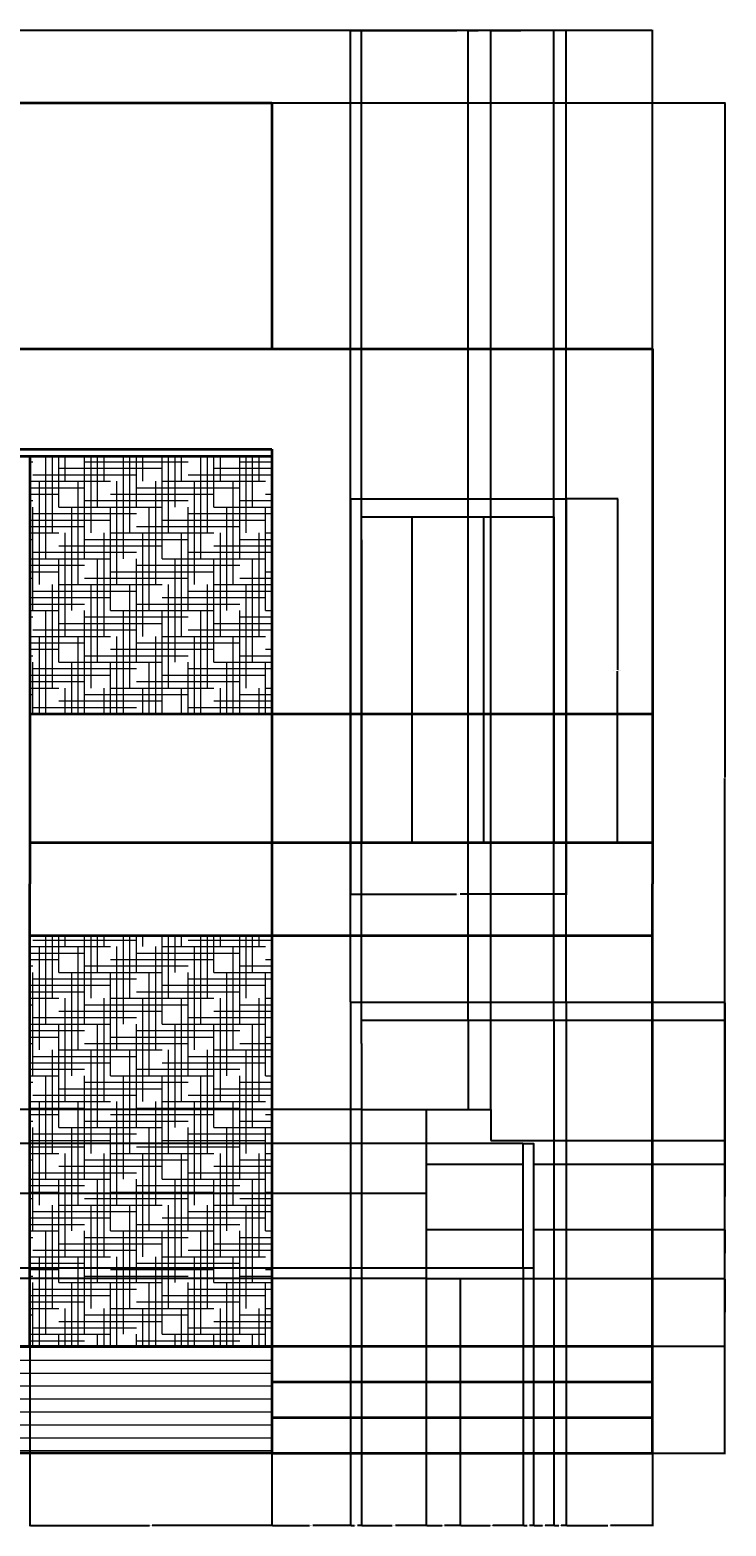
# Model space of a CAD drawing. Units: inches. Extents: x 18 to 448, y 19 to 438.
# Tile 2 of 2: x 253 to 448, y 19 to 438. Entities that reach past the tile are written whole.
import ezdxf

# ---------------------------------------------------------------- set-up
doc = ezdxf.new("R2010")
doc.units = ezdxf.units.IN
doc.header["$MEASUREMENT"] = 0
for name, color, linetype, lineweight in [('A-ANNO-DIMS', 2, 'Continuous', 18), ('A-DOOR', 3, 'Continuous', 25), ('A-ELEV', 7, 'Continuous', 35), ('A-ELEV-PATT', 8, 'Continuous', 13)]:
    doc.layers.add(name, color=color, linetype=linetype, lineweight=lineweight)
doc.styles.get("Standard").update_dxf_attribs({"font": 'arial.ttf'})
doc.dimstyles.get("Standard").update_dxf_attribs({"dimtxt": 0.18, "dimasz": 0.18, "dimexe": 0.18, "dimexo": 0.0625, "dimgap": 0.09, "dimtad": 0, "dimtih": 1, "dimtoh": 1, "dimdec": 4, "dimzin": 0, "dimdsep": 46, "dimtxsty": 'Standard', "dimcen": 0.09, "dimadec": 0, "dimazin": 0, "dimtfac": 1, "dimtdec": 4, "dimtofl": 0, "dimtmove": 0, "dimatfit": 3, "dimfxl": 1, "dimtolj": 1, "dimtzin": 0, "dimarcsym": 0})

# ---------------------------------------------------------------- blocks, each defined once
blk = doc.blocks.new('DOOR-FRAME')
for p, q in [((0, 96.46), (0, 4.77)), ((0, 96.46), (6.57, 96.46)), ((6.57, 96.46), (60.43, 96.46)), ((60.43, 96.46), (60.43, 0)), ((3.01, 84.89), (3.01, 91.39)), ((3.01, 91.39), (57.03, 91.39)), ((57.03, 91.39), (57.03, 84.89)), ((3.01, 84.89), (3.01, 0)), ((57.03, 84.89), (57.03, 0)), ((0, 4.77), (0, 0))]:
    blk.add_line(p, q)
blk = doc.blocks.new('*D5')
at = {"layer": 'A-ANNO-DIMS', "color": 0, "lineweight": -2, "transparency": 16777216}
for p, q in [((403.35, 306.87), (417.94, 306.87)), ((417.76, 306.69), (417.76, 258.82)), ((417.76, 210.58), (417.76, 258.45)), ((403.35, 210.4), (417.94, 210.4))]:
    blk.add_line(p, q, dxfattribs=at)
at = {"layer": 'A-ANNO-DIMS', "color": 0, "transparency": 16777216}
for points in [[(417.73, 306.69), (417.79, 306.69), (417.76, 306.87)], [(417.73, 210.58), (417.79, 210.58), (417.76, 210.4)]]:
    blk.add_solid(points, dxfattribs=at)
at = {"layer": 'Defpoints', "color": 0, "transparency": 16777216}
for p in [(403.29, 306.87), (417.76, 306.87), (403.29, 210.4)]:
    blk.add_point(p, dxfattribs=at)
at = {"layer": 'A-ANNO-DIMS', "color": 0, "transparency": 16777216, "insert": (417.76, 258.64), "char_height": 0.18, "attachment_point": 5}
blk.add_mtext('\\A1;DOOR FRAME 96 TYP.', dxfattribs=at)
blk = doc.blocks.new('*D6')
at = {"layer": 'A-ANNO-DIMS', "color": 0, "lineweight": -2, "transparency": 16777216}
for p, q in [((342.86, 210.34), (342.86, 195.76)), ((403.29, 210.34), (403.29, 195.76)), ((343.04, 195.94), (372.54, 195.94)), ((403.11, 195.94), (373.6, 195.94))]:
    blk.add_line(p, q, dxfattribs=at)
at = {"layer": 'A-ANNO-DIMS', "color": 0, "transparency": 16777216}
for points in [[(343.04, 195.97), (343.04, 195.91), (342.86, 195.94)], [(403.11, 195.97), (403.11, 195.91), (403.29, 195.94)]]:
    blk.add_solid(points, dxfattribs=at)
at = {"layer": 'Defpoints', "color": 0, "transparency": 16777216}
for p in [(342.86, 210.4), (403.29, 210.4), (403.29, 195.94)]:
    blk.add_point(p, dxfattribs=at)
at = {"layer": 'A-ANNO-DIMS', "color": 0, "transparency": 16777216, "insert": (373.07, 195.94), "char_height": 0.18, "attachment_point": 5}
blk.add_mtext('\\A1;60 TYP.', dxfattribs=at)
blk = doc.blocks.new('*D7')
at = {"layer": 'A-ANNO-DIMS', "color": 0, "lineweight": -2, "transparency": 16777216}
for p, q in [((38.85, 39.26), (38.85, 438.34)), ((39.03, 438.16), (232.72, 438.16)), ((427.33, 438.16), (233.64, 438.16)), ((427.51, 39.26), (427.51, 438.34))]:
    blk.add_line(p, q, dxfattribs=at)
at = {"layer": 'A-ANNO-DIMS', "color": 0, "transparency": 16777216}
for points in [[(39.03, 438.19), (39.03, 438.13), (38.85, 438.16)], [(427.33, 438.19), (427.33, 438.13), (427.51, 438.16)]]:
    blk.add_solid(points, dxfattribs=at)
at = {"layer": 'Defpoints', "color": 0, "transparency": 16777216}
for p in [(427.51, 438.16), (38.85, 39.19), (427.51, 39.19)]:
    blk.add_point(p, dxfattribs=at)
at = {"layer": 'A-ANNO-DIMS', "color": 0, "transparency": 16777216, "insert": (233.18, 438.16), "char_height": 0.18, "attachment_point": 5}
blk.add_mtext('\\A1;388.66', dxfattribs=at)
blk = doc.blocks.new('*D8')
at = {"layer": 'A-ANNO-DIMS', "color": 0, "lineweight": -2, "transparency": 16777216}
for p, q in [((320.8, 417.86), (447.99, 417.86)), ((447.81, 417.68), (447.81, 228.71)), ((447.81, 39.37), (447.81, 228.34)), ((427.57, 39.19), (447.99, 39.19))]:
    blk.add_line(p, q, dxfattribs=at)
at = {"layer": 'A-ANNO-DIMS', "color": 0, "transparency": 16777216}
for points in [[(447.78, 417.68), (447.84, 417.68), (447.81, 417.86)], [(447.78, 39.37), (447.84, 39.37), (447.81, 39.19)]]:
    blk.add_solid(points, dxfattribs=at)
at = {"layer": 'Defpoints', "color": 0, "transparency": 16777216}
for p in [(320.74, 417.86), (447.81, 417.86), (427.51, 39.19)]:
    blk.add_point(p, dxfattribs=at)
at = {"layer": 'A-ANNO-DIMS', "color": 0, "transparency": 16777216, "insert": (447.81, 228.52), "char_height": 0.18, "attachment_point": 5}
blk.add_mtext('\\A1;378.66', dxfattribs=at)
blk = doc.blocks.new('*D12')
at = {"layer": 'A-ANNO-DIMS', "color": 0, "lineweight": -2, "transparency": 16777216}
for p, q in [((252.9, 69.13), (252.9, 18.71)), ((320.74, 69.13), (320.74, 18.71)), ((253.08, 18.89), (286.43, 18.89)), ((320.56, 18.89), (287.21, 18.89))]:
    blk.add_line(p, q, dxfattribs=at)
at = {"layer": 'A-ANNO-DIMS', "color": 0, "transparency": 16777216}
for points in [[(253.08, 18.92), (253.08, 18.86), (252.9, 18.89)], [(320.56, 18.92), (320.56, 18.86), (320.74, 18.89)]]:
    blk.add_solid(points, dxfattribs=at)
at = {"layer": 'Defpoints', "color": 0, "transparency": 16777216}
for p in [(252.9, 69.19), (320.74, 69.19), (320.74, 18.89)]:
    blk.add_point(p, dxfattribs=at)
at = {"layer": 'A-ANNO-DIMS', "color": 0, "transparency": 16777216, "insert": (286.82, 18.89), "char_height": 0.18, "attachment_point": 5}
blk.add_mtext('\\A1;67.83', dxfattribs=at)
blk = doc.blocks.new('*D13')
at = {"layer": 'A-ANNO-DIMS', "color": 0, "lineweight": -2, "transparency": 16777216}
for p, q in [((320.74, 69.13), (320.74, 18.71)), ((342.86, 69.13), (342.86, 18.71)), ((320.92, 18.89), (331.33, 18.89)), ((342.68, 18.89), (332.26, 18.89))]:
    blk.add_line(p, q, dxfattribs=at)
at = {"layer": 'A-ANNO-DIMS', "color": 0, "transparency": 16777216}
for points in [[(320.92, 18.92), (320.92, 18.86), (320.74, 18.89)], [(342.68, 18.92), (342.68, 18.86), (342.86, 18.89)]]:
    blk.add_solid(points, dxfattribs=at)
at = {"layer": 'Defpoints', "color": 0, "transparency": 16777216}
for p in [(320.74, 69.19), (342.86, 69.19), (342.86, 18.89)]:
    blk.add_point(p, dxfattribs=at)
at = {"layer": 'A-ANNO-DIMS', "color": 0, "transparency": 16777216, "insert": (331.8, 18.89), "char_height": 0.18, "attachment_point": 5}
blk.add_mtext('\\A1;22.124', dxfattribs=at)
blk = doc.blocks.new('*D14')
at = {"layer": 'A-ANNO-DIMS', "color": 0, "lineweight": -2, "transparency": 16777216}
for p, q in [((403.29, 69.13), (403.29, 18.71)), ((427.51, 69.13), (427.51, 18.71)), ((403.47, 18.89), (415, 18.89)), ((427.33, 18.89), (415.79, 18.89))]:
    blk.add_line(p, q, dxfattribs=at)
at = {"layer": 'A-ANNO-DIMS', "color": 0, "transparency": 16777216}
for points in [[(403.47, 18.92), (403.47, 18.86), (403.29, 18.89)], [(427.33, 18.92), (427.33, 18.86), (427.51, 18.89)]]:
    blk.add_solid(points, dxfattribs=at)
at = {"layer": 'Defpoints', "color": 0, "transparency": 16777216}
for p in [(403.29, 69.19), (427.51, 69.19), (427.51, 18.89)]:
    blk.add_point(p, dxfattribs=at)
at = {"layer": 'A-ANNO-DIMS', "color": 0, "transparency": 16777216, "insert": (415.4, 18.89), "char_height": 0.18, "attachment_point": 5}
blk.add_mtext('\\A1;24.22', dxfattribs=at)
blk = doc.blocks.new('*D24')
at = {"layer": 'A-ANNO-DIMS', "color": 0, "lineweight": -2, "transparency": 16777216}
for p, q in [((345.87, 160.65), (345.87, 438.34)), ((346.05, 438.16), (360.44, 438.16)), ((375.62, 438.16), (361.23, 438.16)), ((375.8, 160.65), (375.8, 438.34))]:
    blk.add_line(p, q, dxfattribs=at)
at = {"layer": 'A-ANNO-DIMS', "color": 0, "transparency": 16777216}
for points in [[(346.05, 438.19), (346.05, 438.13), (345.87, 438.16)], [(375.62, 438.19), (375.62, 438.13), (375.8, 438.16)]]:
    blk.add_solid(points, dxfattribs=at)
at = {"layer": 'Defpoints', "color": 0, "transparency": 16777216}
for p in [(375.8, 438.16), (345.87, 160.58), (375.8, 160.58)]:
    blk.add_point(p, dxfattribs=at)
at = {"layer": 'A-ANNO-DIMS', "color": 0, "transparency": 16777216, "insert": (360.84, 438.16), "char_height": 0.18, "attachment_point": 5}
blk.add_mtext('\\A1;29.93', dxfattribs=at)
blk = doc.blocks.new('*D25')
at = {"layer": 'A-ANNO-DIMS', "color": 0, "lineweight": -2, "transparency": 16777216}
for p, q in [((375.8, 160.65), (375.8, 438.34)), ((375.98, 438.16), (378.63, 438.16)), ((382.06, 438.16), (379.42, 438.16)), ((382.24, 160.65), (382.24, 438.34))]:
    blk.add_line(p, q, dxfattribs=at)
at = {"layer": 'A-ANNO-DIMS', "color": 0, "transparency": 16777216}
for points in [[(375.98, 438.19), (375.98, 438.13), (375.8, 438.16)], [(382.06, 438.19), (382.06, 438.13), (382.24, 438.16)]]:
    blk.add_solid(points, dxfattribs=at)
at = {"layer": 'Defpoints', "color": 0, "transparency": 16777216}
for p in [(382.24, 438.16), (375.8, 160.58), (382.24, 160.58)]:
    blk.add_point(p, dxfattribs=at)
at = {"layer": 'A-ANNO-DIMS', "color": 0, "transparency": 16777216, "insert": (379.02, 438.16), "char_height": 0.18, "attachment_point": 5}
blk.add_mtext('\\A1;6.436', dxfattribs=at)
blk = doc.blocks.new('*D26')
at = {"layer": 'A-ANNO-DIMS', "color": 0, "lineweight": -2, "transparency": 16777216}
for p, q in [((382.24, 160.65), (382.24, 438.34)), ((382.42, 438.16), (390.61, 438.16)), ((399.71, 438.16), (391.52, 438.16)), ((399.89, 160.65), (399.89, 438.34))]:
    blk.add_line(p, q, dxfattribs=at)
at = {"layer": 'A-ANNO-DIMS', "color": 0, "transparency": 16777216}
for points in [[(382.42, 438.19), (382.42, 438.13), (382.24, 438.16)], [(399.71, 438.19), (399.71, 438.13), (399.89, 438.16)]]:
    blk.add_solid(points, dxfattribs=at)
at = {"layer": 'Defpoints', "color": 0, "transparency": 16777216}
for p in [(399.89, 438.16), (382.24, 160.58), (399.89, 160.58)]:
    blk.add_point(p, dxfattribs=at)
at = {"layer": 'A-ANNO-DIMS', "color": 0, "transparency": 16777216, "insert": (391.07, 438.16), "char_height": 0.18, "attachment_point": 5}
blk.add_mtext('\\A1;17.655', dxfattribs=at)
blk = doc.blocks.new('*D27')
at = {"layer": 'A-ANNO-DIMS', "color": 0, "lineweight": -2, "transparency": 16777216}
for p, q in [((342.86, 165.72), (342.86, 438.34)), ((343.04, 438.16), (372.68, 438.16)), ((403.11, 438.16), (373.47, 438.16)), ((403.29, 165.72), (403.29, 438.34))]:
    blk.add_line(p, q, dxfattribs=at)
at = {"layer": 'A-ANNO-DIMS', "color": 0, "transparency": 16777216}
for points in [[(343.04, 438.19), (343.04, 438.13), (342.86, 438.16)], [(403.11, 438.19), (403.11, 438.13), (403.29, 438.16)]]:
    blk.add_solid(points, dxfattribs=at)
at = {"layer": 'Defpoints', "color": 0, "transparency": 16777216}
for p in [(403.29, 438.16), (342.86, 165.66), (403.29, 165.66)]:
    blk.add_point(p, dxfattribs=at)
at = {"layer": 'A-ANNO-DIMS', "color": 0, "transparency": 16777216, "insert": (373.07, 438.16), "char_height": 0.18, "attachment_point": 5}
blk.add_mtext('\\A1;60.43', dxfattribs=at)
blk = doc.blocks.new('*D28')
at = {"layer": 'A-ANNO-DIMS', "color": 0, "lineweight": -2, "transparency": 16777216}
for p, q in [((342.86, 69.13), (342.86, 18.71)), ((345.87, 69.13), (345.87, 18.71)), ((343.04, 18.89), (343.97, 18.89)), ((345.69, 18.89), (344.76, 18.89))]:
    blk.add_line(p, q, dxfattribs=at)
at = {"layer": 'A-ANNO-DIMS', "color": 0, "transparency": 16777216}
for points in [[(343.04, 18.92), (343.04, 18.86), (342.86, 18.89)], [(345.69, 18.92), (345.69, 18.86), (345.87, 18.89)]]:
    blk.add_solid(points, dxfattribs=at)
at = {"layer": 'Defpoints', "color": 0, "transparency": 16777216}
for p in [(342.86, 69.19), (345.87, 69.19), (345.87, 18.89)]:
    blk.add_point(p, dxfattribs=at)
at = {"layer": 'A-ANNO-DIMS', "color": 0, "transparency": 16777216, "insert": (344.37, 18.89), "char_height": 0.18, "attachment_point": 5}
blk.add_mtext('\\A1;3.014', dxfattribs=at)
blk = doc.blocks.new('*D29')
at = {"layer": 'A-ANNO-DIMS', "color": 0, "lineweight": -2, "transparency": 16777216}
for p, q in [((345.87, 88.07), (345.87, 18.71)), ((364.06, 88.07), (364.06, 18.71)), ((346.05, 18.89), (354.51, 18.89)), ((363.88, 18.89), (355.42, 18.89))]:
    blk.add_line(p, q, dxfattribs=at)
at = {"layer": 'A-ANNO-DIMS', "color": 0, "transparency": 16777216}
for points in [[(346.05, 18.92), (346.05, 18.86), (345.87, 18.89)], [(363.88, 18.92), (363.88, 18.86), (364.06, 18.89)]]:
    blk.add_solid(points, dxfattribs=at)
at = {"layer": 'Defpoints', "color": 0, "transparency": 16777216}
for p in [(345.87, 88.13), (364.06, 88.13), (364.06, 18.89)]:
    blk.add_point(p, dxfattribs=at)
at = {"layer": 'A-ANNO-DIMS', "color": 0, "transparency": 16777216, "insert": (354.96, 18.89), "char_height": 0.18, "attachment_point": 5}
blk.add_mtext('\\A1;18.183', dxfattribs=at)
blk = doc.blocks.new('*D30')
at = {"layer": 'A-ANNO-DIMS', "color": 0, "lineweight": -2, "transparency": 16777216}
for p, q in [((364.06, 88.07), (364.06, 18.71)), ((373.61, 88.07), (373.61, 18.71)), ((364.24, 18.89), (368.51, 18.89)), ((373.43, 18.89), (369.16, 18.89))]:
    blk.add_line(p, q, dxfattribs=at)
at = {"layer": 'A-ANNO-DIMS', "color": 0, "transparency": 16777216}
for points in [[(364.24, 18.92), (364.24, 18.86), (364.06, 18.89)], [(373.43, 18.92), (373.43, 18.86), (373.61, 18.89)]]:
    blk.add_solid(points, dxfattribs=at)
at = {"layer": 'Defpoints', "color": 0, "transparency": 16777216}
for p in [(364.06, 88.13), (373.61, 88.13), (373.61, 18.89)]:
    blk.add_point(p, dxfattribs=at)
at = {"layer": 'A-ANNO-DIMS', "color": 0, "transparency": 16777216, "insert": (368.83, 18.89), "char_height": 0.18, "attachment_point": 5}
blk.add_mtext('\\A1;9.55', dxfattribs=at)
blk = doc.blocks.new('*D31')
at = {"layer": 'A-ANNO-DIMS', "color": 0, "lineweight": -2, "transparency": 16777216}
for p, q in [((391.23, 91.03), (391.23, 18.71)), ((373.61, 88.07), (373.61, 18.71)), ((373.79, 18.89), (382.03, 18.89)), ((391.05, 18.89), (382.8, 18.89))]:
    blk.add_line(p, q, dxfattribs=at)
at = {"layer": 'A-ANNO-DIMS', "color": 0, "transparency": 16777216}
for points in [[(373.79, 18.92), (373.79, 18.86), (373.61, 18.89)], [(391.05, 18.92), (391.05, 18.86), (391.23, 18.89)]]:
    blk.add_solid(points, dxfattribs=at)
at = {"layer": 'Defpoints', "color": 0, "transparency": 16777216}
for p in [(373.61, 88.13), (391.23, 91.09), (391.23, 18.89)]:
    blk.add_point(p, dxfattribs=at)
at = {"layer": 'A-ANNO-DIMS', "color": 0, "transparency": 16777216, "insert": (382.42, 18.89), "char_height": 0.18, "attachment_point": 5}
blk.add_mtext('\\A1;17.62', dxfattribs=at)
blk = doc.blocks.new('*D32')
at = {"layer": 'A-ANNO-DIMS', "color": 0, "lineweight": -2, "transparency": 16777216}
for p, q in [((391.23, 91.03), (391.23, 18.71)), ((394.18, 91.03), (394.18, 18.71)), ((391.41, 18.89), (392.37, 18.89)), ((394, 18.89), (393.03, 18.89))]:
    blk.add_line(p, q, dxfattribs=at)
at = {"layer": 'A-ANNO-DIMS', "color": 0, "transparency": 16777216}
for points in [[(391.41, 18.92), (391.41, 18.86), (391.23, 18.89)], [(394, 18.92), (394, 18.86), (394.18, 18.89)]]:
    blk.add_solid(points, dxfattribs=at)
at = {"layer": 'Defpoints', "color": 0, "transparency": 16777216}
for p in [(391.23, 91.09), (394.18, 91.09), (394.18, 18.89)]:
    blk.add_point(p, dxfattribs=at)
at = {"layer": 'A-ANNO-DIMS', "color": 0, "transparency": 16777216, "insert": (392.7, 18.89), "char_height": 0.18, "attachment_point": 5}
blk.add_mtext('\\A1;2.95', dxfattribs=at)
blk = doc.blocks.new('*D33')
at = {"layer": 'A-ANNO-DIMS', "color": 0, "lineweight": -2, "transparency": 16777216}
for p, q in [((394.18, 91.03), (394.18, 18.71)), ((399.89, 69.13), (399.89, 18.71)), ((394.36, 18.89), (396.64, 18.89)), ((399.71, 18.89), (397.43, 18.89))]:
    blk.add_line(p, q, dxfattribs=at)
at = {"layer": 'A-ANNO-DIMS', "color": 0, "transparency": 16777216}
for points in [[(394.36, 18.92), (394.36, 18.86), (394.18, 18.89)], [(399.71, 18.92), (399.71, 18.86), (399.89, 18.89)]]:
    blk.add_solid(points, dxfattribs=at)
at = {"layer": 'Defpoints', "color": 0, "transparency": 16777216}
for p in [(394.18, 91.09), (399.89, 69.19), (399.89, 18.89)]:
    blk.add_point(p, dxfattribs=at)
at = {"layer": 'A-ANNO-DIMS', "color": 0, "transparency": 16777216, "insert": (397.03, 18.89), "char_height": 0.18, "attachment_point": 5}
blk.add_mtext('\\A1;5.719', dxfattribs=at)
blk = doc.blocks.new('*D34')
at = {"layer": 'A-ANNO-DIMS', "color": 0, "lineweight": -2, "transparency": 16777216}
for p, q in [((399.89, 69.13), (399.89, 18.71)), ((403.29, 69.13), (403.29, 18.71)), ((400.07, 18.89), (401.27, 18.89)), ((403.11, 18.89), (401.91, 18.89))]:
    blk.add_line(p, q, dxfattribs=at)
at = {"layer": 'A-ANNO-DIMS', "color": 0, "transparency": 16777216}
for points in [[(400.07, 18.92), (400.07, 18.86), (399.89, 18.89)], [(403.11, 18.92), (403.11, 18.86), (403.29, 18.89)]]:
    blk.add_solid(points, dxfattribs=at)
at = {"layer": 'Defpoints', "color": 0, "transparency": 16777216}
for p in [(399.89, 69.19), (403.29, 69.19), (403.29, 18.89)]:
    blk.add_point(p, dxfattribs=at)
at = {"layer": 'A-ANNO-DIMS', "color": 0, "transparency": 16777216, "insert": (401.59, 18.89), "char_height": 0.18, "attachment_point": 5}
blk.add_mtext('\\A1;3.39', dxfattribs=at)
blk = doc.blocks.new('*D35')
at = {"layer": 'A-ANNO-DIMS', "color": 0, "lineweight": -2, "transparency": 16777216}
for p, q in [((399.96, 88.13), (447.99, 88.13)), ((447.81, 87.95), (447.81, 78.84)), ((447.81, 69.37), (447.81, 78.48)), ((399.96, 69.19), (447.99, 69.19))]:
    blk.add_line(p, q, dxfattribs=at)
at = {"layer": 'A-ANNO-DIMS', "color": 0, "transparency": 16777216}
for points in [[(447.78, 87.95), (447.84, 87.95), (447.81, 88.13)], [(447.78, 69.37), (447.84, 69.37), (447.81, 69.19)]]:
    blk.add_solid(points, dxfattribs=at)
at = {"layer": 'Defpoints', "color": 0, "transparency": 16777216}
for p in [(399.89, 88.13), (447.81, 88.13), (399.89, 69.19)]:
    blk.add_point(p, dxfattribs=at)
at = {"layer": 'A-ANNO-DIMS', "color": 0, "transparency": 16777216, "insert": (447.81, 78.66), "char_height": 0.18, "attachment_point": 5}
blk.add_mtext('\\A1;18.934', dxfattribs=at)
blk = doc.blocks.new('*D36')
at = {"layer": 'A-ANNO-DIMS', "color": 0, "lineweight": -2, "transparency": 16777216}
for p, q in [((399.96, 101.94), (447.99, 101.94)), ((447.81, 101.76), (447.81, 95.22)), ((447.81, 88.31), (447.81, 94.85)), ((399.96, 88.13), (447.99, 88.13))]:
    blk.add_line(p, q, dxfattribs=at)
at = {"layer": 'A-ANNO-DIMS', "color": 0, "transparency": 16777216}
for points in [[(447.78, 101.76), (447.84, 101.76), (447.81, 101.94)], [(447.78, 88.31), (447.84, 88.31), (447.81, 88.13)]]:
    blk.add_solid(points, dxfattribs=at)
at = {"layer": 'Defpoints', "color": 0, "transparency": 16777216}
for p in [(399.89, 101.94), (447.81, 101.94), (399.89, 88.13)]:
    blk.add_point(p, dxfattribs=at)
at = {"layer": 'A-ANNO-DIMS', "color": 0, "transparency": 16777216, "insert": (447.81, 95.03), "char_height": 0.18, "attachment_point": 5}
blk.add_mtext('\\A1;13.812', dxfattribs=at)
blk = doc.blocks.new('*D37')
at = {"layer": 'A-ANNO-DIMS', "color": 0, "lineweight": -2, "transparency": 16777216}
for p, q in [((399.96, 120.24), (447.99, 120.24)), ((447.81, 120.06), (447.81, 111.27)), ((447.81, 102.12), (447.81, 110.91)), ((399.96, 101.94), (447.99, 101.94))]:
    blk.add_line(p, q, dxfattribs=at)
at = {"layer": 'A-ANNO-DIMS', "color": 0, "transparency": 16777216}
for points in [[(447.78, 120.06), (447.84, 120.06), (447.81, 120.24)], [(447.78, 102.12), (447.84, 102.12), (447.81, 101.94)]]:
    blk.add_solid(points, dxfattribs=at)
at = {"layer": 'Defpoints', "color": 0, "transparency": 16777216}
for p in [(399.89, 120.24), (447.81, 120.24), (399.89, 101.94)]:
    blk.add_point(p, dxfattribs=at)
at = {"layer": 'A-ANNO-DIMS', "color": 0, "transparency": 16777216, "insert": (447.81, 111.09), "char_height": 0.18, "attachment_point": 5}
blk.add_mtext('\\A1;18.297', dxfattribs=at)
blk = doc.blocks.new('*D38')
at = {"layer": 'A-ANNO-DIMS', "color": 0, "lineweight": -2, "transparency": 16777216}
for p, q in [((399.96, 126.88), (447.99, 126.88)), ((447.81, 126.7), (447.81, 123.74)), ((447.81, 120.42), (447.81, 123.38)), ((399.96, 120.24), (447.99, 120.24))]:
    blk.add_line(p, q, dxfattribs=at)
at = {"layer": 'A-ANNO-DIMS', "color": 0, "transparency": 16777216}
for points in [[(447.78, 126.7), (447.84, 126.7), (447.81, 126.88)], [(447.78, 120.42), (447.84, 120.42), (447.81, 120.24)]]:
    blk.add_solid(points, dxfattribs=at)
at = {"layer": 'Defpoints', "color": 0, "transparency": 16777216}
for p in [(399.89, 126.88), (447.81, 126.88), (399.89, 120.24)]:
    blk.add_point(p, dxfattribs=at)
at = {"layer": 'A-ANNO-DIMS', "color": 0, "transparency": 16777216, "insert": (447.81, 123.56), "char_height": 0.18, "attachment_point": 5}
blk.add_mtext('\\A1;6.644', dxfattribs=at)
blk = doc.blocks.new('*D39')
at = {"layer": 'A-ANNO-DIMS', "color": 0, "lineweight": -2, "transparency": 16777216}
for p, q in [((399.96, 160.58), (447.99, 160.58)), ((447.81, 160.4), (447.81, 143.91)), ((447.81, 127.06), (447.81, 143.55)), ((399.96, 126.88), (447.99, 126.88))]:
    blk.add_line(p, q, dxfattribs=at)
at = {"layer": 'A-ANNO-DIMS', "color": 0, "transparency": 16777216}
for points in [[(447.78, 160.4), (447.84, 160.4), (447.81, 160.58)], [(447.78, 127.06), (447.84, 127.06), (447.81, 126.88)]]:
    blk.add_solid(points, dxfattribs=at)
at = {"layer": 'Defpoints', "color": 0, "transparency": 16777216}
for p in [(399.89, 160.58), (447.81, 160.58), (399.89, 126.88)]:
    blk.add_point(p, dxfattribs=at)
at = {"layer": 'A-ANNO-DIMS', "color": 0, "transparency": 16777216, "insert": (447.81, 143.73), "char_height": 0.18, "attachment_point": 5}
blk.add_mtext('\\A1;33.7', dxfattribs=at)
blk = doc.blocks.new('*D40')
at = {"layer": 'A-ANNO-DIMS', "color": 0, "lineweight": -2, "transparency": 16777216}
for p, q in [((403.35, 165.66), (447.99, 165.66)), ((447.81, 165.48), (447.81, 163.3)), ((399.96, 160.58), (447.99, 160.58)), ((447.81, 160.76), (447.81, 162.94))]:
    blk.add_line(p, q, dxfattribs=at)
at = {"layer": 'A-ANNO-DIMS', "color": 0, "transparency": 16777216}
for points in [[(447.78, 165.48), (447.84, 165.48), (447.81, 165.66)], [(447.78, 160.76), (447.84, 160.76), (447.81, 160.58)]]:
    blk.add_solid(points, dxfattribs=at)
at = {"layer": 'Defpoints', "color": 0, "transparency": 16777216}
for p in [(403.29, 165.66), (447.81, 165.66), (399.89, 160.58)]:
    blk.add_point(p, dxfattribs=at)
at = {"layer": 'A-ANNO-DIMS', "color": 0, "transparency": 16777216, "insert": (447.81, 163.12), "char_height": 0.18, "attachment_point": 5}
blk.add_mtext('\\A1;5.071', dxfattribs=at)
blk = doc.blocks.new('*D41')
at = {"layer": 'A-ANNO-DIMS', "color": 0, "lineweight": -2, "transparency": 16777216}
for p, q in [((403.35, 165.66), (447.99, 165.66)), ((447.81, 165.48), (447.81, 117.61)), ((447.81, 69.37), (447.81, 117.24)), ((403.35, 69.19), (447.99, 69.19))]:
    blk.add_line(p, q, dxfattribs=at)
at = {"layer": 'A-ANNO-DIMS', "color": 0, "transparency": 16777216}
for points in [[(447.78, 165.48), (447.84, 165.48), (447.81, 165.66)], [(447.78, 69.37), (447.84, 69.37), (447.81, 69.19)]]:
    blk.add_solid(points, dxfattribs=at)
at = {"layer": 'Defpoints', "color": 0, "transparency": 16777216}
for p in [(403.29, 165.66), (447.81, 165.66), (403.29, 69.19)]:
    blk.add_point(p, dxfattribs=at)
at = {"layer": 'A-ANNO-DIMS', "color": 0, "transparency": 16777216, "insert": (447.81, 117.42), "char_height": 0.18, "attachment_point": 5}
blk.add_mtext('\\A1;96.46', dxfattribs=at)
blk = doc.blocks.new('*D42')
at = {"layer": 'A-ANNO-DIMS', "color": 0, "lineweight": -2, "transparency": 16777216}
for p, q in [((345.81, 111.98), (18.37, 111.98)), ((18.55, 111.8), (18.55, 100.23)), ((18.55, 88.31), (18.55, 99.87)), ((345.81, 88.13), (18.37, 88.13))]:
    blk.add_line(p, q, dxfattribs=at)
at = {"layer": 'A-ANNO-DIMS', "color": 0, "transparency": 16777216}
for points in [[(18.52, 111.8), (18.58, 111.8), (18.55, 111.98)], [(18.52, 88.31), (18.58, 88.31), (18.55, 88.13)]]:
    blk.add_solid(points, dxfattribs=at)
at = {"layer": 'Defpoints', "color": 0, "transparency": 16777216}
for p in [(18.55, 111.98), (345.87, 111.98), (345.87, 88.13)]:
    blk.add_point(p, dxfattribs=at)
at = {"layer": 'A-ANNO-DIMS', "color": 0, "transparency": 16777216, "insert": (18.55, 100.05), "char_height": 0.18, "attachment_point": 5}
blk.add_mtext('\\A1;23.85', dxfattribs=at)
blk = doc.blocks.new('*D43')
at = {"layer": 'A-ANNO-DIMS', "color": 0, "lineweight": -2, "transparency": 16777216}
for p, q in [((345.81, 135.54), (18.37, 135.54)), ((18.55, 135.36), (18.55, 123.94)), ((18.55, 112.16), (18.55, 123.58)), ((345.81, 111.98), (18.37, 111.98))]:
    blk.add_line(p, q, dxfattribs=at)
at = {"layer": 'A-ANNO-DIMS', "color": 0, "transparency": 16777216}
for points in [[(18.52, 135.36), (18.58, 135.36), (18.55, 135.54)], [(18.52, 112.16), (18.58, 112.16), (18.55, 111.98)]]:
    blk.add_solid(points, dxfattribs=at)
at = {"layer": 'Defpoints', "color": 0, "transparency": 16777216}
for p in [(18.55, 135.54), (345.87, 135.54), (345.87, 111.98)]:
    blk.add_point(p, dxfattribs=at)
at = {"layer": 'A-ANNO-DIMS', "color": 0, "transparency": 16777216, "insert": (18.55, 123.76), "char_height": 0.18, "attachment_point": 5}
blk.add_mtext('\\A1;23.56', dxfattribs=at)
blk = doc.blocks.new('*D44')
at = {"layer": 'A-ANNO-DIMS', "color": 0, "lineweight": -2, "transparency": 16777216}
for p, q in [((391.16, 91.09), (18.37, 91.09)), ((18.55, 90.91), (18.55, 80.33)), ((18.55, 69.37), (18.55, 79.96)), ((373.54, 69.19), (18.37, 69.19))]:
    blk.add_line(p, q, dxfattribs=at)
at = {"layer": 'A-ANNO-DIMS', "color": 0, "transparency": 16777216}
for points in [[(18.52, 90.91), (18.58, 90.91), (18.55, 91.09)], [(18.52, 69.37), (18.58, 69.37), (18.55, 69.19)]]:
    blk.add_solid(points, dxfattribs=at)
at = {"layer": 'Defpoints', "color": 0, "transparency": 16777216}
for p in [(18.55, 91.09), (391.23, 91.09), (373.61, 69.19)]:
    blk.add_point(p, dxfattribs=at)
at = {"layer": 'A-ANNO-DIMS', "color": 0, "transparency": 16777216, "insert": (18.55, 80.14), "char_height": 0.18, "attachment_point": 5}
blk.add_mtext('\\A1;21.9', dxfattribs=at)
blk = doc.blocks.new('*D45')
at = {"layer": 'A-ANNO-DIMS', "color": 0, "lineweight": -2, "transparency": 16777216}
for p, q in [((391.16, 125.99), (18.37, 125.99)), ((18.55, 125.81), (18.55, 108.73)), ((18.55, 91.27), (18.55, 108.36)), ((391.16, 91.09), (18.37, 91.09))]:
    blk.add_line(p, q, dxfattribs=at)
at = {"layer": 'A-ANNO-DIMS', "color": 0, "transparency": 16777216}
for points in [[(18.52, 125.81), (18.58, 125.81), (18.55, 125.99)], [(18.52, 91.27), (18.58, 91.27), (18.55, 91.09)]]:
    blk.add_solid(points, dxfattribs=at)
at = {"layer": 'Defpoints', "color": 0, "transparency": 16777216}
for p in [(18.55, 125.99), (391.23, 125.99), (391.23, 91.09)]:
    blk.add_point(p, dxfattribs=at)
at = {"layer": 'A-ANNO-DIMS', "color": 0, "transparency": 16777216, "insert": (18.55, 108.54), "char_height": 0.18, "attachment_point": 5}
blk.add_mtext('\\A1;34.9', dxfattribs=at)

msp = doc.modelspace()

# ---------------------------------------------------------------- hatches: boundary and pattern name
at = {"layer": 'A-ELEV-PATT'}
h = msp.add_hatch(dxfattribs=at)
h.set_pattern_fill('HOUND', color=256, scale=29)
h.paths.add_polyline_path([(320.7354, 318.796), (252.9033, 318.796), (252.9033, 246.4909), (320.7354, 246.4909)])
h.paths.add_polyline_path([(320.7354, 184.3438), (252.9033, 184.3438), (252.9033, 69.1939), (320.7354, 69.1939)])
h = msp.add_hatch(dxfattribs=at)
h.set_pattern_fill('ANSI31', color=256, scale=29, angle=135)
h.paths.add_polyline_path([(320.7354, 59.1939), (320.7354, 69.1939), (38.8517, 69.1939), (38.8517, 39.1939), (320.7354, 39.1939), (320.7354, 49.1939)])

# ---------------------------------------------------------------- linework, layer by layer
at = {"layer": 'A-DOOR'}
for p, q in [((360.0186, 301.795), (360.0186, 210.4047)), ((380.1238, 301.795), (380.1238, 210.4047)), ((375.8032, 160.5843), (375.8032, 135.5385)), ((382.2391, 135.5385), (382.2391, 160.5843)), ((345.8731, 135.5385), (382.2391, 135.5385)), ((364.0561, 135.5385), (364.0561, 111.9775)), ((382.2391, 135.5385), (382.2391, 126.8811)), ((382.2391, 126.8811), (399.8938, 126.8811)), ((364.0561, 120.2367), (391.2265, 120.2367)), ((394.1751, 120.2367), (399.8938, 120.2367)), ((364.0561, 111.9775), (345.8731, 111.9775)), ((364.0561, 111.9775), (364.0561, 101.9397)), ((364.0561, 101.9397), (391.2265, 101.9397)), ((364.0561, 101.9397), (364.0561, 88.1277)), ((394.1751, 101.9397), (399.8938, 101.9397)), ((364.0561, 88.1277), (345.8731, 88.1277)), ((364.0561, 88.1277), (399.8938, 88.1277)), ((373.6066, 88.1277), (373.6066, 69.1939))]:
    msp.add_line(p, q, dxfattribs=at)
msp.add_lwpolyline([(391.2265, 125.9945), (394.1751, 125.9945), (394.1751, 91.0931), (391.2265, 91.0931)], close=True, dxfattribs=at)
at = {"layer": 'A-ELEV'}
for p, q in [((92.2414, 417.8553), (320.7354, 417.8553)), ((320.7354, 417.8553), (320.7354, 348.9241)), ((92.2414, 348.9241), (427.508, 348.9241)), ((427.508, 348.9241), (427.508, 198.796)), ((92.2414, 320.796), (252.9033, 320.796)), ((252.9033, 320.796), (320.7354, 320.796)), ((320.7354, 320.796), (320.7354, 318.796)), ((92.2414, 318.796), (252.9033, 318.796)), ((252.9033, 318.796), (252.9033, 198.796)), ((252.9033, 318.796), (320.7354, 318.796)), ((320.7354, 318.796), (320.7354, 198.796)), ((252.9033, 246.4909), (427.508, 246.4909)), ((252.9033, 210.4047), (427.508, 210.4047)), ((252.9033, 69.1939), (252.9033, 198.796)), ((320.7354, 198.796), (320.7354, 69.1939)), ((427.508, 69.1939), (427.508, 198.796)), ((252.9033, 184.3438), (427.508, 184.3438)), ((38.8517, 69.1939), (427.508, 69.1939)), ((320.7354, 69.1939), (320.7354, 59.1939)), ((427.508, 59.1939), (427.508, 69.1939)), ((320.7354, 59.1939), (427.508, 59.1939)), ((320.7354, 59.1939), (320.7354, 49.1939)), ((427.508, 49.1939), (427.508, 59.1939)), ((320.7354, 49.1939), (427.508, 49.1939)), ((320.7354, 49.1939), (320.7354, 39.1939)), ((427.508, 39.1939), (427.508, 49.1939)), ((320.7354, 39.1939), (38.8517, 39.1939)), ((320.7354, 39.1939), (427.508, 39.1939))]:
    msp.add_line(p, q, dxfattribs=at)

# ---------------------------------------------------------------- block references
at = {"layer": 'A-DOOR'}
for p in [(342.859, 210.4047), (342.859, 69.194)]:
    msp.add_blockref('DOOR-FRAME', p, dxfattribs=at)

# ---------------------------------------------------------------- dimensions: what is measured, and where the dimension line sits
at = {"layer": 'A-ANNO-DIMS'}
for base, p1, p2, override, picture, middle in [((427.508, 438.1553), (38.8517, 39.1939), (427.508, 39.1939), {"dimdec": 2, "dimlfac": 1, "dimrnd": 0, "dimzin": 0, "dimdsep": 46, "dimlunit": 2}, '*D7', (233.1799, 438.1553)), ((403.2874, 438.1553), (342.8594, 165.6556), (403.2874, 165.6556), {"dimdec": 2, "dimlfac": 1, "dimrnd": 0, "dimzin": 0, "dimdsep": 46, "dimlunit": 2}, '*D27', (373.0734, 438.1553)), ((375.8032, 438.1553), (345.8731, 160.5843), (375.8032, 160.5843), {"dimdec": 2, "dimlfac": 1, "dimrnd": 0, "dimzin": 0, "dimdsep": 46, "dimlunit": 2}, '*D24', (360.8382, 438.1553)), ((382.2391, 438.1553), (375.8032, 160.5843), (382.2391, 160.5843), {"dimdec": 3, "dimlfac": 1, "dimrnd": 0, "dimzin": 0, "dimdsep": 46, "dimlunit": 2}, '*D25', (379.0211, 438.1553)), ((399.8938, 438.1553), (382.2391, 160.5843), (399.8938, 160.5843), {"dimdec": 3, "dimlfac": 1, "dimrnd": 0, "dimzin": 0, "dimdsep": 46, "dimlunit": 2}, '*D26', (391.0665, 438.1553)), ((364.0561, 18.8939), (345.8731, 88.1277), (364.0561, 88.1277), {"dimdec": 3, "dimlfac": 1, "dimrnd": 0, "dimzin": 0, "dimdsep": 46, "dimlunit": 2}, '*D29', (354.9646, 18.8939)), ((373.6066, 18.8939), (364.0561, 88.1277), (373.6066, 88.1277), {"dimdec": 2, "dimlfac": 1, "dimrnd": 0, "dimzin": 0, "dimdsep": 46, "dimlunit": 2}, '*D30', (368.8314, 18.8939)), ((391.2265, 18.8939), (373.6066, 88.1277), (391.2265, 91.0931), {"dimdec": 2, "dimlfac": 1, "dimrnd": 0, "dimzin": 0, "dimdsep": 46, "dimlunit": 2}, '*D31', (382.4166, 18.8939)), ((394.1751, 18.8939), (391.2265, 91.0931), (394.1751, 91.0931), {"dimdec": 2, "dimlfac": 1, "dimrnd": 0, "dimzin": 0, "dimdsep": 46, "dimlunit": 2}, '*D32', (392.7008, 18.8939)), ((399.8938, 18.8939), (394.1751, 91.0931), (399.8938, 69.1939), {"dimdec": 3, "dimlfac": 1, "dimrnd": 0, "dimzin": 0, "dimdsep": 46, "dimlunit": 2}, '*D33', (397.0345, 18.8939)), ((320.7354, 18.8939), (252.9033, 69.1939), (320.7354, 69.1939), {"dimdec": 2, "dimlfac": 1, "dimrnd": 0, "dimzin": 0, "dimdsep": 46, "dimlunit": 2}, '*D12', (286.8193, 18.8939)), ((342.8594, 18.8939), (320.7354, 69.1939), (342.8594, 69.1939), {"dimdec": 3, "dimlfac": 1, "dimrnd": 0, "dimzin": 0, "dimdsep": 46, "dimlunit": 2}, '*D13', (331.7974, 18.8939)), ((345.8731, 18.8939), (342.8594, 69.1939), (345.8731, 69.1939), {"dimdec": 3, "dimlfac": 1, "dimrnd": 0, "dimzin": 0, "dimdsep": 46, "dimlunit": 2}, '*D28', (344.3663, 18.8939)), ((403.2874, 18.8939), (399.8938, 69.1939), (403.2874, 69.1939), {"dimdec": 2, "dimlfac": 1, "dimrnd": 0, "dimzin": 0, "dimdsep": 46, "dimlunit": 2}, '*D34', (401.5906, 18.8939)), ((427.508, 18.8939), (403.2874, 69.1939), (427.508, 69.1939), {"dimdec": 2, "dimlfac": 1, "dimrnd": 0, "dimzin": 0, "dimdsep": 46, "dimlunit": 2}, '*D14', (415.3977, 18.8939))]:
    dim = msp.add_linear_dim(base=base, p1=p1, p2=p2, dimstyle='Standard', override=override, dxfattribs=at)
    dim.commit()
    dim.dimension.update_dxf_attribs({"geometry": picture, "text_midpoint": middle})
for base, p1, p2, override, picture, middle in [((447.808, 417.8553), (427.508, 39.1939), (320.7354, 417.8553), {"dimdec": 2, "dimlfac": 1, "dimrnd": 0, "dimzin": 0, "dimdsep": 46, "dimlunit": 2}, '*D8', (447.808, 228.5246)), ((447.808, 165.6556), (399.8938, 160.5843), (403.2874, 165.6556), {"dimdec": 3, "dimlfac": 1, "dimrnd": 0, "dimzin": 0, "dimdsep": 46, "dimlunit": 2}, '*D40', (447.808, 163.1199)), ((447.808, 165.6556), (403.2874, 69.1939), (403.2874, 165.6556), {"dimdec": 2, "dimlfac": 1, "dimrnd": 0, "dimzin": 0, "dimdsep": 46, "dimlunit": 2}, '*D41', (447.808, 117.4247)), ((447.808, 160.5843), (399.8938, 126.8811), (399.8938, 160.5843), {"dimdec": 1, "dimlfac": 1, "dimrnd": 0, "dimzin": 0, "dimdsep": 46, "dimlunit": 2}, '*D39', (447.808, 143.7327)), ((18.5517, 135.5385), (345.8731, 111.9775), (345.8731, 135.5385), {"dimdec": 2, "dimlfac": 1, "dimrnd": 0, "dimzin": 0, "dimdsep": 46, "dimlunit": 2}, '*D43', (18.5517, 123.758)), ((18.5517, 125.9945), (391.2265, 91.0931), (391.2265, 125.9945), {"dimdec": 1, "dimlfac": 1, "dimrnd": 0, "dimzin": 0, "dimdsep": 46, "dimlunit": 2}, '*D45', (18.5517, 108.5438)), ((447.808, 126.8811), (399.8938, 120.2367), (399.8938, 126.8811), {"dimdec": 3, "dimlfac": 1, "dimrnd": 0, "dimzin": 0, "dimdsep": 46, "dimlunit": 2}, '*D38', (447.808, 123.5589)), ((447.808, 120.2367), (399.8938, 101.9397), (399.8938, 120.2367), {"dimdec": 3, "dimlfac": 1, "dimrnd": 0, "dimzin": 0, "dimdsep": 46, "dimlunit": 2}, '*D37', (447.808, 111.0882)), ((18.5517, 111.9775), (345.8731, 88.1277), (345.8731, 111.9775), {"dimdec": 2, "dimlfac": 1, "dimrnd": 0, "dimzin": 0, "dimdsep": 46, "dimlunit": 2}, '*D42', (18.5517, 100.0526)), ((447.808, 101.9397), (399.8938, 88.1277), (399.8938, 101.9397), {"dimdec": 3, "dimlfac": 1, "dimrnd": 0, "dimzin": 0, "dimdsep": 46, "dimlunit": 2}, '*D36', (447.808, 95.0337)), ((18.5517, 91.0931), (373.6066, 69.1939), (391.2265, 91.0931), {"dimdec": 1, "dimlfac": 1, "dimrnd": 0, "dimzin": 0, "dimdsep": 46, "dimlunit": 2}, '*D44', (18.5517, 80.1435)), ((447.808, 88.1277), (399.8938, 69.1939), (399.8938, 88.1277), {"dimdec": 3, "dimlfac": 1, "dimrnd": 0, "dimzin": 0, "dimdsep": 46, "dimlunit": 2}, '*D35', (447.808, 78.6608))]:
    dim = msp.add_linear_dim(base=base, p1=p1, p2=p2, angle=90, dimstyle='Standard', override=override, dxfattribs=at)
    dim.commit()
    dim.dimension.update_dxf_attribs({"geometry": picture, "text_midpoint": middle})
dim = msp.add_linear_dim(base=(417.7566, 306.8663), p1=(403.2874, 210.4047), p2=(403.2874, 306.8663), angle=90, text='DOOR FRAME <> TYP.', dimstyle='Standard', override={"dimdec": 0, "dimlfac": 1, "dimrnd": 0, "dimzin": 0, "dimdsep": 46, "dimlunit": 2}, dxfattribs=at)
dim.commit()
dim.dimension.update_dxf_attribs({"geometry": '*D5', "text_midpoint": (417.7566, 258.6355)})
dim = msp.add_linear_dim(base=(403.2874, 195.9354), p1=(342.8594, 210.4047), p2=(403.2874, 210.4047), text='<> TYP.', dimstyle='Standard', override={"dimdec": 0, "dimlfac": 1, "dimrnd": 0, "dimzin": 0, "dimdsep": 46, "dimlunit": 2}, dxfattribs=at)
dim.commit()
dim.dimension.update_dxf_attribs({"geometry": '*D6', "text_midpoint": (373.0734, 195.9354)})

doc.saveas('drawing.dxf')
